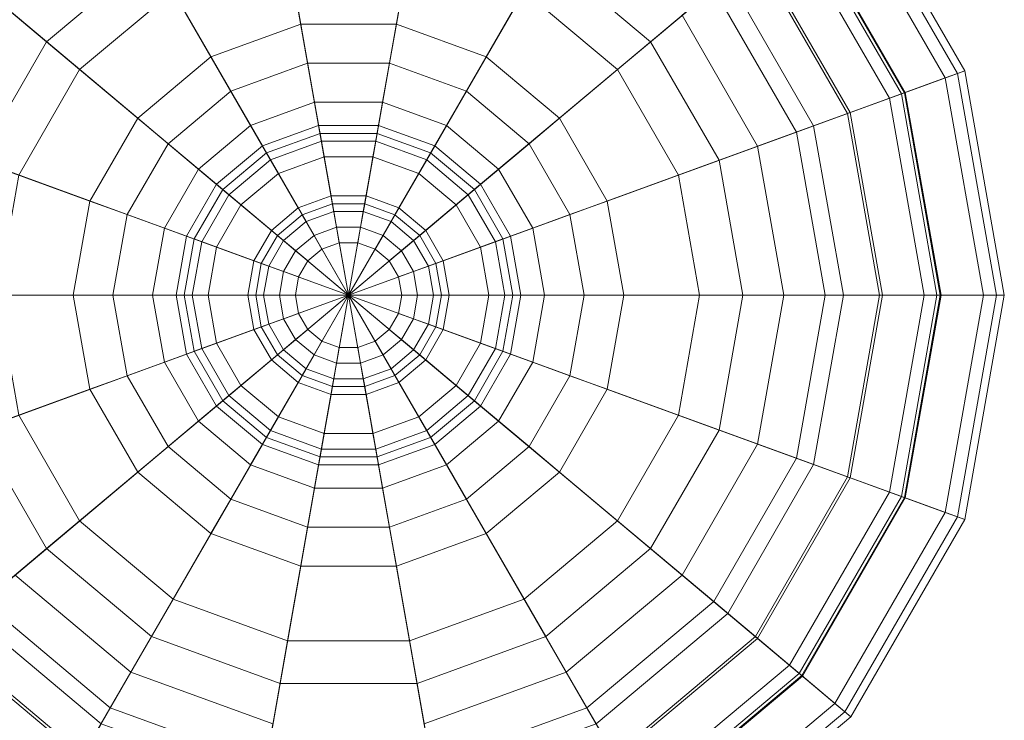
# Model space of a CAD drawing. Units: inches. Extents: x 375 to 1122, y 27 to 1069.
# Tile 22 of 155: x 718.584 to 720.617, y 272.362 to 273.809. Entities that reach past the tile are written whole.
import ezdxf

# ---------------------------------------------------------------- set-up
doc = ezdxf.new("R2010")
doc.units = ezdxf.units.IN
doc.layers.add('Furniture', color=30, linetype='Continuous', lineweight=18)

# ---------------------------------------------------------------- blocks, each defined once
blk = doc.blocks.new('A$C403C54AD')
for points in [[(1.826559, 0.891746, -0.031825), (1.826559, 0.857884, -0.028747), (1.826559, 0.857884, -0.028747), (1.814977, 0.889704, -0.031825)], [(1.826559, 0.88848, -0.028594), (1.826559, 0.891746, -0.031825), (1.814977, 0.889704, -0.031825), (1.816094, 0.886635, -0.028594)], [(1.826559, 0.88844, 0.131159), (1.826559, 0.891347, 0.117935), (1.815114, 0.889329, 0.117935), (1.816108, 0.886597, 0.131159)], [(1.826559, 0.891347, 0.117935), (1.826559, 0.890672, 0.089693), (1.815345, 0.888695, 0.089693), (1.815114, 0.889329, 0.117935)], [(1.83814, 0.889704, -0.031825), (1.826559, 0.857884, -0.028747), (1.826559, 0.857884, -0.028747), (1.826559, 0.891746, -0.031825)], [(1.837023, 0.886635, -0.028594), (1.83814, 0.889704, -0.031825), (1.826559, 0.891746, -0.031825), (1.826559, 0.88848, -0.028594)], [(1.83701, 0.886597, 0.131159), (1.838004, 0.889329, 0.117935), (1.826559, 0.891347, 0.117935), (1.826559, 0.88844, 0.131159)], [(1.838004, 0.889329, 0.117935), (1.837773, 0.888695, 0.089693), (1.826559, 0.890672, 0.089693), (1.826559, 0.891347, 0.117935)], [(1.826559, 0.890672, 0.089693), (1.826559, 0.885308, 0.071684), (1.817179, 0.883654, 0.071684), (1.815345, 0.888695, 0.089693)], [(1.837773, 0.888695, 0.089693), (1.835938, 0.883654, 0.071684), (1.826559, 0.885308, 0.071684), (1.826559, 0.890672, 0.089693)], [(1.816094, 0.886635, -0.028594), (1.814977, 0.889704, -0.031825), (1.804793, 0.883824, -0.031825), (1.806892, 0.881322, -0.028594)], [(1.814977, 0.889704, -0.031825), (1.826559, 0.857884, -0.028747), (1.826559, 0.857884, -0.028747), (1.804793, 0.883824, -0.031825)], [(1.816108, 0.886597, 0.131159), (1.815114, 0.889329, 0.117935), (1.805049, 0.883518, 0.117935), (1.806918, 0.881291, 0.131159)], [(1.815114, 0.889329, 0.117935), (1.815345, 0.888695, 0.089693), (1.805483, 0.883001, 0.089693), (1.805049, 0.883518, 0.117935)], [(1.848325, 0.883824, -0.031825), (1.826559, 0.857884, -0.028747), (1.826559, 0.857884, -0.028747), (1.83814, 0.889704, -0.031825)], [(1.8462, 0.881291, 0.131159), (1.848069, 0.883518, 0.117935), (1.838004, 0.889329, 0.117935), (1.83701, 0.886597, 0.131159)], [(1.846226, 0.881322, -0.028594), (1.848325, 0.883824, -0.031825), (1.83814, 0.889704, -0.031825), (1.837023, 0.886635, -0.028594)], [(1.848069, 0.883518, 0.117935), (1.847635, 0.883001, 0.089693), (1.837773, 0.888695, 0.089693), (1.838004, 0.889329, 0.117935)], [(1.815345, 0.888695, 0.089693), (1.817179, 0.883654, 0.071684), (1.808931, 0.878892, 0.071684), (1.805483, 0.883001, 0.089693)], [(1.826559, 0.872098, -0.02532), (1.826559, 0.88848, -0.028594), (1.816094, 0.886635, -0.028594), (1.821697, 0.871241, -0.02532)], [(1.826559, 0.883444, 0.140564), (1.826559, 0.88844, 0.131159), (1.816108, 0.886597, 0.131159), (1.817817, 0.881902, 0.140564)], [(1.826559, 0.888263, 0.117718), (1.826559, 0.885453, 0.130354), (1.81713, 0.88379, 0.130354), (1.816169, 0.886431, 0.117718)], [(1.826559, 0.887605, 0.090178), (1.826559, 0.888263, 0.117718), (1.816169, 0.886431, 0.117718), (1.816394, 0.885812, 0.090178)], [(1.83142, 0.871241, -0.02532), (1.837023, 0.886635, -0.028594), (1.826559, 0.88848, -0.028594), (1.826559, 0.872098, -0.02532)], [(1.835301, 0.881902, 0.140564), (1.83701, 0.886597, 0.131159), (1.826559, 0.88844, 0.131159), (1.826559, 0.883444, 0.140564)], [(1.836949, 0.886431, 0.117718), (1.835988, 0.88379, 0.130354), (1.826559, 0.885453, 0.130354), (1.826559, 0.888263, 0.117718)], [(1.836724, 0.885812, 0.090178), (1.836949, 0.886431, 0.117718), (1.826559, 0.888263, 0.117718), (1.826559, 0.887605, 0.090178)], [(1.847635, 0.883001, 0.089693), (1.844187, 0.878892, 0.071684), (1.835938, 0.883654, 0.071684), (1.837773, 0.888695, 0.089693)], [(1.826559, 0.882497, 0.073031), (1.826559, 0.887605, 0.090178), (1.816394, 0.885812, 0.090178), (1.818141, 0.881013, 0.073031)], [(1.834977, 0.881013, 0.073031), (1.836724, 0.885812, 0.090178), (1.826559, 0.887605, 0.090178), (1.826559, 0.882497, 0.073031)], [(1.821697, 0.871241, -0.02532), (1.816094, 0.886635, -0.028594), (1.806892, 0.881322, -0.028594), (1.817422, 0.868773, -0.02532)], [(1.817817, 0.881902, 0.140564), (1.816108, 0.886597, 0.131159), (1.806918, 0.881291, 0.131159), (1.81013, 0.877464, 0.140564)], [(1.816169, 0.886431, 0.117718), (1.81713, 0.88379, 0.130354), (1.808838, 0.879003, 0.130354), (1.807032, 0.881156, 0.117718)], [(1.816394, 0.885812, 0.090178), (1.816169, 0.886431, 0.117718), (1.807032, 0.881156, 0.117718), (1.807455, 0.880651, 0.090178)], [(1.835696, 0.868773, -0.02532), (1.846226, 0.881322, -0.028594), (1.837023, 0.886635, -0.028594), (1.83142, 0.871241, -0.02532)], [(1.842988, 0.877464, 0.140564), (1.8462, 0.881291, 0.131159), (1.83701, 0.886597, 0.131159), (1.835301, 0.881902, 0.140564)], [(1.846086, 0.881156, 0.117718), (1.84428, 0.879003, 0.130354), (1.835988, 0.88379, 0.130354), (1.836949, 0.886431, 0.117718)], [(1.845663, 0.880651, 0.090178), (1.846086, 0.881156, 0.117718), (1.836949, 0.886431, 0.117718), (1.836724, 0.885812, 0.090178)], [(1.818141, 0.881013, 0.073031), (1.816394, 0.885812, 0.090178), (1.807455, 0.880651, 0.090178), (1.810738, 0.876739, 0.073031)], [(1.84238, 0.876739, 0.073031), (1.845663, 0.880651, 0.090178), (1.836724, 0.885812, 0.090178), (1.834977, 0.881013, 0.073031)], [(1.826559, 0.885453, 0.130354), (1.826559, 0.880365, 0.140564), (1.81887, 0.879009, 0.140564), (1.81713, 0.88379, 0.130354)], [(1.826559, 0.885308, 0.071684), (1.826559, 0.878242, 0.061451), (1.819596, 0.877014, 0.061451), (1.817179, 0.883654, 0.071684)], [(1.835988, 0.88379, 0.130354), (1.834248, 0.879009, 0.140564), (1.826559, 0.880365, 0.140564), (1.826559, 0.885453, 0.130354)], [(1.835938, 0.883654, 0.071684), (1.833522, 0.877014, 0.061451), (1.826559, 0.878242, 0.061451), (1.826559, 0.885308, 0.071684)], [(1.804793, 0.883824, -0.031825), (1.826559, 0.857884, -0.028747), (1.826559, 0.857884, -0.028747), (1.797233, 0.874815, -0.031825)], [(1.81713, 0.88379, 0.130354), (1.81887, 0.879009, 0.140564), (1.812108, 0.875106, 0.140564), (1.808838, 0.879003, 0.130354)], [(1.855884, 0.874815, -0.031825), (1.826559, 0.857884, -0.028747), (1.826559, 0.857884, -0.028747), (1.848325, 0.883824, -0.031825)], [(1.84428, 0.879003, 0.130354), (1.84101, 0.875106, 0.140564), (1.834248, 0.879009, 0.140564), (1.835988, 0.88379, 0.130354)], [(1.853056, 0.873182, -0.028594), (1.855884, 0.874815, -0.031825), (1.848325, 0.883824, -0.031825), (1.846226, 0.881322, -0.028594)], [(1.817179, 0.883654, 0.071684), (1.819596, 0.877014, 0.061451), (1.813473, 0.873479, 0.061451), (1.808931, 0.878892, 0.071684)], [(1.826559, 0.880365, 0.140564), (1.826559, 0.883444, 0.140564), (1.817817, 0.881902, 0.140564), (1.81887, 0.879009, 0.140564)], [(1.834248, 0.879009, 0.140564), (1.835301, 0.881902, 0.140564), (1.826559, 0.883444, 0.140564), (1.826559, 0.880365, 0.140564)], [(1.844187, 0.878892, 0.071684), (1.839644, 0.873479, 0.061451), (1.833522, 0.877014, 0.061451), (1.835938, 0.883654, 0.071684)], [(1.853021, 0.873162, 0.131159), (1.855539, 0.874616, 0.117935), (1.848069, 0.883518, 0.117935), (1.8462, 0.881291, 0.131159)], [(1.855539, 0.874616, 0.117935), (1.854954, 0.874278, 0.089693), (1.847635, 0.883001, 0.089693), (1.848069, 0.883518, 0.117935)], [(1.854954, 0.874278, 0.089693), (1.850309, 0.871596, 0.071684), (1.844187, 0.878892, 0.071684), (1.847635, 0.883001, 0.089693)], [(1.826559, 0.876011, 0.063639), (1.826559, 0.882497, 0.073031), (1.818141, 0.881013, 0.073031), (1.820359, 0.874918, 0.063639)], [(1.832759, 0.874918, 0.063639), (1.834977, 0.881013, 0.073031), (1.826559, 0.882497, 0.073031), (1.826559, 0.876011, 0.063639)], [(1.81887, 0.879009, 0.140564), (1.817817, 0.881902, 0.140564), (1.81013, 0.877464, 0.140564), (1.812108, 0.875106, 0.140564)], [(1.84101, 0.875106, 0.140564), (1.842988, 0.877464, 0.140564), (1.835301, 0.881902, 0.140564), (1.834248, 0.879009, 0.140564)], [(1.817422, 0.868773, -0.02532), (1.806892, 0.881322, -0.028594), (1.800062, 0.873182, -0.028594), (1.814249, 0.864991, -0.02532)], [(1.838869, 0.864991, -0.02532), (1.853056, 0.873182, -0.028594), (1.846226, 0.881322, -0.028594), (1.835696, 0.868773, -0.02532)], [(1.848694, 0.870664, 0.140564), (1.853021, 0.873162, 0.131159), (1.8462, 0.881291, 0.131159), (1.842988, 0.877464, 0.140564)], [(1.852868, 0.873073, 0.117718), (1.850434, 0.871669, 0.130354), (1.84428, 0.879003, 0.130354), (1.846086, 0.881156, 0.117718)], [(1.852298, 0.872744, 0.090178), (1.852868, 0.873073, 0.117718), (1.846086, 0.881156, 0.117718), (1.845663, 0.880651, 0.090178)], [(1.820359, 0.874918, 0.063639), (1.818141, 0.881013, 0.073031), (1.810738, 0.876739, 0.073031), (1.814907, 0.87177, 0.063639)], [(1.838211, 0.87177, 0.063639), (1.84238, 0.876739, 0.073031), (1.834977, 0.881013, 0.073031), (1.832759, 0.874918, 0.063639)], [(1.847874, 0.87019, 0.073031), (1.852298, 0.872744, 0.090178), (1.845663, 0.880651, 0.090178), (1.84238, 0.876739, 0.073031)], [(1.808931, 0.878892, 0.071684), (1.813473, 0.873479, 0.061451), (1.808929, 0.868063, 0.061451), (1.802809, 0.871596, 0.071684)], [(1.850309, 0.871596, 0.071684), (1.844189, 0.868063, 0.061451), (1.839644, 0.873479, 0.061451), (1.844187, 0.878892, 0.071684)], [(1.850434, 0.871669, 0.130354), (1.846028, 0.869125, 0.140564), (1.84101, 0.875106, 0.140564), (1.84428, 0.879003, 0.130354)], [(1.826559, 0.878242, 0.061451), (1.826559, 0.868003, 0.054084), (1.823098, 0.867392, 0.054084), (1.819596, 0.877014, 0.061451)], [(1.833522, 0.877014, 0.061451), (1.83002, 0.867392, 0.054084), (1.826559, 0.868003, 0.054084), (1.826559, 0.878242, 0.061451)], [(1.846028, 0.869125, 0.140564), (1.848694, 0.870664, 0.140564), (1.842988, 0.877464, 0.140564), (1.84101, 0.875106, 0.140564)], [(1.814907, 0.87177, 0.063639), (1.810738, 0.876739, 0.073031), (1.805243, 0.87019, 0.073031), (1.81086, 0.866948, 0.063639)], [(1.819596, 0.877014, 0.061451), (1.823098, 0.867392, 0.054084), (1.820055, 0.865635, 0.054084), (1.813473, 0.873479, 0.061451)], [(1.839644, 0.873479, 0.061451), (1.833063, 0.865635, 0.054084), (1.83002, 0.867392, 0.054084), (1.833522, 0.877014, 0.061451)], [(1.842258, 0.866948, 0.063639), (1.847874, 0.87019, 0.073031), (1.84238, 0.876739, 0.073031), (1.838211, 0.87177, 0.063639)], [(1.826559, 0.866788, 0.057003), (1.826559, 0.876011, 0.063639), (1.820359, 0.874918, 0.063639), (1.823514, 0.866251, 0.057003)], [(1.829604, 0.866251, 0.057003), (1.832759, 0.874918, 0.063639), (1.826559, 0.876011, 0.063639), (1.826559, 0.866788, 0.057003)], [(1.797233, 0.874815, -0.031825), (1.826559, 0.857884, -0.028747), (1.826559, 0.857884, -0.028747), (1.793211, 0.863764, -0.031825)], [(1.823514, 0.866251, 0.057003), (1.820359, 0.874918, 0.063639), (1.814907, 0.87177, 0.063639), (1.820835, 0.864705, 0.057003)], [(1.859907, 0.863764, -0.031825), (1.826559, 0.857884, -0.028747), (1.826559, 0.857884, -0.028747), (1.855884, 0.874815, -0.031825)], [(1.832282, 0.864705, 0.057003), (1.838211, 0.87177, 0.063639), (1.832759, 0.874918, 0.063639), (1.829604, 0.866251, 0.057003)], [(1.814249, 0.864991, -0.02532), (1.800062, 0.873182, -0.028594), (1.796427, 0.863197, -0.028594), (1.812561, 0.860352, -0.02532)], [(1.813473, 0.873479, 0.061451), (1.820055, 0.865635, 0.054084), (1.817796, 0.862943, 0.054084), (1.808929, 0.868063, 0.061451)], [(1.844189, 0.868063, 0.061451), (1.835322, 0.862943, 0.054084), (1.833063, 0.865635, 0.054084), (1.839644, 0.873479, 0.061451)], [(1.840557, 0.860352, -0.02532), (1.85669, 0.863197, -0.028594), (1.853056, 0.873182, -0.028594), (1.838869, 0.864991, -0.02532)], [(1.850798, 0.862158, 0.073031), (1.855828, 0.863045, 0.090178), (1.852298, 0.872744, 0.090178), (1.847874, 0.87019, 0.073031)], [(1.826559, 0.87005, -0.022455), (1.826559, 0.872098, -0.02532), (1.821697, 0.871241, -0.02532), (1.822398, 0.869317, -0.022455)], [(1.83072, 0.869317, -0.022455), (1.83142, 0.871241, -0.02532), (1.826559, 0.872098, -0.02532), (1.826559, 0.87005, -0.022455)], [(1.820835, 0.864705, 0.057003), (1.814907, 0.87177, 0.063639), (1.81086, 0.866948, 0.063639), (1.818848, 0.862336, 0.057003)], [(1.83427, 0.862336, 0.057003), (1.842258, 0.866948, 0.063639), (1.838211, 0.87177, 0.063639), (1.832282, 0.864705, 0.057003)], [(1.853566, 0.862646, 0.071684), (1.846607, 0.861419, 0.061451), (1.844189, 0.868063, 0.061451), (1.850309, 0.871596, 0.071684)], [(1.853709, 0.862671, 0.130354), (1.848699, 0.861788, 0.140564), (1.846028, 0.869125, 0.140564), (1.850434, 0.871669, 0.130354)], [(1.822398, 0.869317, -0.022455), (1.821697, 0.871241, -0.02532), (1.817422, 0.868773, -0.02532), (1.818738, 0.867204, -0.022455)], [(1.834379, 0.867204, -0.022455), (1.835696, 0.868773, -0.02532), (1.83142, 0.871241, -0.02532), (1.83072, 0.869317, -0.022455)], [(1.848699, 0.861788, 0.140564), (1.85173, 0.862322, 0.140564), (1.848694, 0.870664, 0.140564), (1.846028, 0.869125, 0.140564)], [(1.826559, 0.865955, -0.020408), (1.826559, 0.87005, -0.022455), (1.822398, 0.869317, -0.022455), (1.823798, 0.865468, -0.020408)], [(1.829319, 0.865468, -0.020408), (1.83072, 0.869317, -0.022455), (1.826559, 0.87005, -0.022455), (1.826559, 0.865955, -0.020408)], [(1.844411, 0.861032, 0.063639), (1.850798, 0.862158, 0.073031), (1.847874, 0.87019, 0.073031), (1.842258, 0.866948, 0.063639)], [(1.823798, 0.865468, -0.020408), (1.822398, 0.869317, -0.022455), (1.818738, 0.867204, -0.022455), (1.821371, 0.864067, -0.020408)], [(1.831747, 0.864067, -0.020408), (1.834379, 0.867204, -0.022455), (1.83072, 0.869317, -0.022455), (1.829319, 0.865468, -0.020408)], [(1.818738, 0.867204, -0.022455), (1.817422, 0.868773, -0.02532), (1.814249, 0.864991, -0.02532), (1.816022, 0.863967, -0.022455)], [(1.837095, 0.863967, -0.022455), (1.838869, 0.864991, -0.02532), (1.835696, 0.868773, -0.02532), (1.834379, 0.867204, -0.022455)], [(1.808929, 0.868063, 0.061451), (1.817796, 0.862943, 0.054084), (1.816594, 0.859641, 0.054084), (1.806511, 0.861419, 0.061451)], [(1.826559, 0.868003, 0.054084), (1.826559, 0.863088, 0.053266), (1.824779, 0.862774, 0.053266), (1.823098, 0.867392, 0.054084)], [(1.83002, 0.867392, 0.054084), (1.828339, 0.862774, 0.053266), (1.826559, 0.863088, 0.053266), (1.826559, 0.868003, 0.054084)], [(1.846607, 0.861419, 0.061451), (1.836524, 0.859641, 0.054084), (1.835322, 0.862943, 0.054084), (1.844189, 0.868063, 0.061451)], [(1.818848, 0.862336, 0.057003), (1.81086, 0.866948, 0.063639), (1.808707, 0.861032, 0.063639), (1.81779, 0.85943, 0.057003)], [(1.821371, 0.864067, -0.020408), (1.818738, 0.867204, -0.022455), (1.816022, 0.863967, -0.022455), (1.819569, 0.861919, -0.020408)], [(1.823098, 0.867392, 0.054084), (1.824779, 0.862774, 0.053266), (1.823214, 0.861871, 0.053266), (1.820055, 0.865635, 0.054084)], [(1.833063, 0.865635, 0.054084), (1.829904, 0.861871, 0.053266), (1.828339, 0.862774, 0.053266), (1.83002, 0.867392, 0.054084)], [(1.833549, 0.861919, -0.020408), (1.837095, 0.863967, -0.022455), (1.834379, 0.867204, -0.022455), (1.831747, 0.864067, -0.020408)], [(1.835328, 0.85943, 0.057003), (1.844411, 0.861032, 0.063639), (1.842258, 0.866948, 0.063639), (1.83427, 0.862336, 0.057003)], [(1.826559, 0.857884, 0.055519), (1.826559, 0.866788, 0.057003), (1.823514, 0.866251, 0.057003), (1.826559, 0.857884, 0.055519)], [(1.826559, 0.857884, 0.055519), (1.829604, 0.866251, 0.057003), (1.826559, 0.866788, 0.057003), (1.826559, 0.857884, 0.055519)], [(1.826559, 0.857884, 0.055519), (1.823514, 0.866251, 0.057003), (1.820835, 0.864705, 0.057003), (1.826559, 0.857884, 0.055519)], [(1.826559, 0.866365, 0.0504), (1.826559, 0.862269, 0.048354), (1.825059, 0.862005, 0.048354), (1.823658, 0.865853, 0.0504)], [(1.826559, 0.865136, 0.052447), (1.826559, 0.866365, 0.0504), (1.823658, 0.865853, 0.0504), (1.824079, 0.864699, 0.052447)], [(1.826559, 0.862679, -0.015087), (1.826559, 0.865955, -0.020408), (1.823798, 0.865468, -0.020408), (1.824919, 0.862389, -0.015087)], [(1.829459, 0.865853, 0.0504), (1.828059, 0.862005, 0.048354), (1.826559, 0.862269, 0.048354), (1.826559, 0.866365, 0.0504)], [(1.829039, 0.864699, 0.052447), (1.829459, 0.865853, 0.0504), (1.826559, 0.866365, 0.0504), (1.826559, 0.865136, 0.052447)], [(1.826559, 0.857884, 0.055519), (1.832282, 0.864705, 0.057003), (1.829604, 0.866251, 0.057003), (1.826559, 0.857884, 0.055519)], [(1.828199, 0.862389, -0.015087), (1.829319, 0.865468, -0.020408), (1.826559, 0.865955, -0.020408), (1.826559, 0.862679, -0.015087)], [(1.820055, 0.865635, 0.054084), (1.823214, 0.861871, 0.053266), (1.822052, 0.860486, 0.053266), (1.817796, 0.862943, 0.054084)], [(1.823658, 0.865853, 0.0504), (1.825059, 0.862005, 0.048354), (1.82374, 0.861243, 0.048354), (1.821108, 0.86438, 0.0504)], [(1.824079, 0.864699, 0.052447), (1.823658, 0.865853, 0.0504), (1.821108, 0.86438, 0.0504), (1.821897, 0.863439, 0.052447)], [(1.824919, 0.862389, -0.015087), (1.823798, 0.865468, -0.020408), (1.821371, 0.864067, -0.020408), (1.823477, 0.861557, -0.015087)], [(1.83201, 0.86438, 0.0504), (1.829378, 0.861243, 0.048354), (1.828059, 0.862005, 0.048354), (1.829459, 0.865853, 0.0504)], [(1.829641, 0.861557, -0.015087), (1.831747, 0.864067, -0.020408), (1.829319, 0.865468, -0.020408), (1.828199, 0.862389, -0.015087)], [(1.83122, 0.863439, 0.052447), (1.83201, 0.86438, 0.0504), (1.829459, 0.865853, 0.0504), (1.829039, 0.864699, 0.052447)], [(1.835322, 0.862943, 0.054084), (1.831066, 0.860486, 0.053266), (1.829904, 0.861871, 0.053266), (1.833063, 0.865635, 0.054084)], [(1.816022, 0.863967, -0.022455), (1.814249, 0.864991, -0.02532), (1.812561, 0.860352, -0.02532), (1.814577, 0.859997, -0.022455)], [(1.826559, 0.863088, 0.053266), (1.826559, 0.865136, 0.052447), (1.824079, 0.864699, 0.052447), (1.824779, 0.862774, 0.053266)], [(1.828339, 0.862774, 0.053266), (1.829039, 0.864699, 0.052447), (1.826559, 0.865136, 0.052447), (1.826559, 0.863088, 0.053266)], [(1.838541, 0.859997, -0.022455), (1.840557, 0.860352, -0.02532), (1.838869, 0.864991, -0.02532), (1.837095, 0.863967, -0.022455)], [(1.826559, 0.857884, 0.055519), (1.820835, 0.864705, 0.057003), (1.818848, 0.862336, 0.057003), (1.826559, 0.857884, 0.055519)], [(1.821108, 0.86438, 0.0504), (1.82374, 0.861243, 0.048354), (1.822761, 0.860076, 0.048354), (1.819215, 0.862124, 0.0504)], [(1.821897, 0.863439, 0.052447), (1.821108, 0.86438, 0.0504), (1.819215, 0.862124, 0.0504), (1.820279, 0.86151, 0.052447)], [(1.824779, 0.862774, 0.053266), (1.824079, 0.864699, 0.052447), (1.821897, 0.863439, 0.052447), (1.823214, 0.861871, 0.053266)], [(1.826559, 0.857884, 0.055519), (1.83427, 0.862336, 0.057003), (1.832282, 0.864705, 0.057003), (1.826559, 0.857884, 0.055519)], [(1.829904, 0.861871, 0.053266), (1.83122, 0.863439, 0.052447), (1.829039, 0.864699, 0.052447), (1.828339, 0.862774, 0.053266)], [(1.833903, 0.862124, 0.0504), (1.830356, 0.860076, 0.048354), (1.829378, 0.861243, 0.048354), (1.83201, 0.86438, 0.0504)], [(1.832839, 0.86151, 0.052447), (1.833903, 0.862124, 0.0504), (1.83201, 0.86438, 0.0504), (1.83122, 0.863439, 0.052447)], [(1.819569, 0.861919, -0.020408), (1.816022, 0.863967, -0.022455), (1.814577, 0.859997, -0.022455), (1.818611, 0.859285, -0.020408)], [(1.823477, 0.861557, -0.015087), (1.821371, 0.864067, -0.020408), (1.819569, 0.861919, -0.020408), (1.822407, 0.860281, -0.015087)], [(1.830711, 0.860281, -0.015087), (1.833549, 0.861919, -0.020408), (1.831747, 0.864067, -0.020408), (1.829641, 0.861557, -0.015087)], [(1.834507, 0.859285, -0.020408), (1.838541, 0.859997, -0.022455), (1.837095, 0.863967, -0.022455), (1.833549, 0.861919, -0.020408)], [(1.793211, 0.863764, -0.031825), (1.826559, 0.857884, -0.028747), (1.826559, 0.857884, -0.028747), (1.793211, 0.852004, -0.031825)], [(1.823214, 0.861871, 0.053266), (1.821897, 0.863439, 0.052447), (1.820279, 0.86151, 0.052447), (1.822052, 0.860486, 0.053266)], [(1.859907, 0.852004, -0.031825), (1.826559, 0.857884, -0.028747), (1.826559, 0.857884, -0.028747), (1.859907, 0.863764, -0.031825)], [(1.831066, 0.860486, 0.053266), (1.832839, 0.86151, 0.052447), (1.83122, 0.863439, 0.052447), (1.829904, 0.861871, 0.053266)], [(1.812561, 0.860352, -0.02532), (1.796427, 0.863197, -0.028594), (1.796427, 0.852571, -0.028594), (1.812561, 0.855416, -0.02532)], [(1.817796, 0.862943, 0.054084), (1.822052, 0.860486, 0.053266), (1.821434, 0.858788, 0.053266), (1.816594, 0.859641, 0.054084)], [(1.836524, 0.859641, 0.054084), (1.831684, 0.858788, 0.053266), (1.831066, 0.860486, 0.053266), (1.835322, 0.862943, 0.054084)], [(1.840557, 0.855416, -0.02532), (1.85669, 0.852571, -0.028594), (1.85669, 0.863197, -0.028594), (1.840557, 0.860352, -0.02532)], [(1.826559, 0.857884, 0.055519), (1.818848, 0.862336, 0.057003), (1.81779, 0.85943, 0.057003), (1.826559, 0.857884, 0.055519)], [(1.825339, 0.861235, -0.006492), (1.824919, 0.862389, -0.015087), (1.823477, 0.861557, -0.015087), (1.824267, 0.860616, -0.006492)], [(1.826559, 0.86145, -0.006492), (1.826559, 0.862679, -0.015087), (1.824919, 0.862389, -0.015087), (1.825339, 0.861235, -0.006492)], [(1.827779, 0.861235, -0.006492), (1.828199, 0.862389, -0.015087), (1.826559, 0.862679, -0.015087), (1.826559, 0.86145, -0.006492)], [(1.826559, 0.857884, 0.055519), (1.835328, 0.85943, 0.057003), (1.83427, 0.862336, 0.057003), (1.826559, 0.857884, 0.055519)], [(1.828851, 0.860616, -0.006492), (1.829641, 0.861557, -0.015087), (1.828199, 0.862389, -0.015087), (1.827779, 0.861235, -0.006492)], [(1.853566, 0.853122, 0.071684), (1.846607, 0.854349, 0.061451), (1.846607, 0.861419, 0.061451), (1.853566, 0.862646, 0.071684)], [(1.820279, 0.86151, 0.052447), (1.819215, 0.862124, 0.0504), (1.818207, 0.859357, 0.0504), (1.819417, 0.859143, 0.052447)], [(1.819215, 0.862124, 0.0504), (1.822761, 0.860076, 0.048354), (1.82224, 0.858645, 0.048354), (1.818207, 0.859357, 0.0504)], [(1.822407, 0.860281, -0.015087), (1.819569, 0.861919, -0.020408), (1.818611, 0.859285, -0.020408), (1.821837, 0.858717, -0.015087)], [(1.825059, 0.862005, 0.048354), (1.825619, 0.860465, 0.041805), (1.824793, 0.859988, 0.041805), (1.82374, 0.861243, 0.048354)], [(1.826559, 0.862269, 0.048354), (1.826559, 0.860631, 0.041805), (1.825619, 0.860465, 0.041805), (1.825059, 0.862005, 0.048354)], [(1.828059, 0.862005, 0.048354), (1.827498, 0.860465, 0.041805), (1.826559, 0.860631, 0.041805), (1.826559, 0.862269, 0.048354)], [(1.829378, 0.861243, 0.048354), (1.828325, 0.859988, 0.041805), (1.827498, 0.860465, 0.041805), (1.828059, 0.862005, 0.048354)], [(1.834911, 0.859357, 0.0504), (1.830877, 0.858645, 0.048354), (1.830356, 0.860076, 0.048354), (1.833903, 0.862124, 0.0504)], [(1.831281, 0.858717, -0.015087), (1.834507, 0.859285, -0.020408), (1.833549, 0.861919, -0.020408), (1.830711, 0.860281, -0.015087)], [(1.833701, 0.859143, 0.052447), (1.834911, 0.859357, 0.0504), (1.833903, 0.862124, 0.0504), (1.832839, 0.86151, 0.052447)], [(1.844411, 0.854736, 0.063639), (1.850798, 0.85361, 0.073031), (1.850798, 0.862158, 0.073031), (1.844411, 0.861032, 0.063639)], [(1.806511, 0.861419, 0.061451), (1.816594, 0.859641, 0.054084), (1.816594, 0.856127, 0.054084), (1.806511, 0.854349, 0.061451)], [(1.822052, 0.860486, 0.053266), (1.820279, 0.86151, 0.052447), (1.819417, 0.859143, 0.052447), (1.821434, 0.858788, 0.053266)], [(1.824267, 0.860616, -0.006492), (1.823477, 0.861557, -0.015087), (1.822407, 0.860281, -0.015087), (1.823471, 0.859667, -0.006492)], [(1.826559, 0.860631, 0.041805), (1.826559, 0.86145, -0.006492), (1.825339, 0.861235, -0.006492), (1.825619, 0.860465, 0.041805)], [(1.827498, 0.860465, 0.041805), (1.827779, 0.861235, -0.006492), (1.826559, 0.86145, -0.006492), (1.826559, 0.860631, 0.041805)], [(1.829647, 0.859667, -0.006492), (1.830711, 0.860281, -0.015087), (1.829641, 0.861557, -0.015087), (1.828851, 0.860616, -0.006492)], [(1.831684, 0.858788, 0.053266), (1.833701, 0.859143, 0.052447), (1.832839, 0.86151, 0.052447), (1.831066, 0.860486, 0.053266)], [(1.846607, 0.854349, 0.061451), (1.836524, 0.856127, 0.054084), (1.836524, 0.859641, 0.054084), (1.846607, 0.861419, 0.061451)], [(1.81779, 0.85943, 0.057003), (1.808707, 0.861032, 0.063639), (1.808707, 0.854736, 0.063639), (1.81779, 0.856338, 0.057003)], [(1.82374, 0.861243, 0.048354), (1.824793, 0.859988, 0.041805), (1.82418, 0.859257, 0.041805), (1.822761, 0.860076, 0.048354)], [(1.825619, 0.860465, 0.041805), (1.825339, 0.861235, -0.006492), (1.824267, 0.860616, -0.006492), (1.824793, 0.859988, 0.041805)], [(1.828325, 0.859988, 0.041805), (1.828851, 0.860616, -0.006492), (1.827779, 0.861235, -0.006492), (1.827498, 0.860465, 0.041805)], [(1.830356, 0.860076, 0.048354), (1.828938, 0.859257, 0.041805), (1.828325, 0.859988, 0.041805), (1.829378, 0.861243, 0.048354)], [(1.835328, 0.856338, 0.057003), (1.844411, 0.854736, 0.063639), (1.844411, 0.861032, 0.063639), (1.835328, 0.85943, 0.057003)], [(1.814577, 0.859997, -0.022455), (1.812561, 0.860352, -0.02532), (1.812561, 0.855416, -0.02532), (1.814577, 0.855771, -0.022455)], [(1.824793, 0.859988, 0.041805), (1.824267, 0.860616, -0.006492), (1.823471, 0.859667, -0.006492), (1.82418, 0.859257, 0.041805)], [(1.828938, 0.859257, 0.041805), (1.829647, 0.859667, -0.006492), (1.828851, 0.860616, -0.006492), (1.828325, 0.859988, 0.041805)], [(1.838541, 0.855771, -0.022455), (1.840557, 0.855416, -0.02532), (1.840557, 0.860352, -0.02532), (1.838541, 0.859997, -0.022455)], [(1.818611, 0.859285, -0.020408), (1.814577, 0.859997, -0.022455), (1.814577, 0.855771, -0.022455), (1.818611, 0.856482, -0.020408)], [(1.823471, 0.859667, -0.006492), (1.822407, 0.860281, -0.015087), (1.821837, 0.858717, -0.015087), (1.823047, 0.858503, -0.006492)], [(1.822761, 0.860076, 0.048354), (1.82418, 0.859257, 0.041805), (1.823854, 0.858361, 0.041805), (1.82224, 0.858645, 0.048354)], [(1.830877, 0.858645, 0.048354), (1.829264, 0.858361, 0.041805), (1.828938, 0.859257, 0.041805), (1.830356, 0.860076, 0.048354)], [(1.830071, 0.858503, -0.006492), (1.831281, 0.858717, -0.015087), (1.830711, 0.860281, -0.015087), (1.829647, 0.859667, -0.006492)], [(1.834507, 0.856482, -0.020408), (1.838541, 0.855771, -0.022455), (1.838541, 0.859997, -0.022455), (1.834507, 0.859285, -0.020408)], [(1.816594, 0.859641, 0.054084), (1.821434, 0.858788, 0.053266), (1.821434, 0.85698, 0.053266), (1.816594, 0.856127, 0.054084)], [(1.826559, 0.857884, 0.055519), (1.81779, 0.85943, 0.057003), (1.81779, 0.856338, 0.057003), (1.826559, 0.857884, 0.055519)], [(1.819417, 0.859143, 0.052447), (1.818207, 0.859357, 0.0504), (1.818207, 0.856411, 0.0504), (1.819417, 0.856625, 0.052447)], [(1.818207, 0.859357, 0.0504), (1.82224, 0.858645, 0.048354), (1.82224, 0.857123, 0.048354), (1.818207, 0.856411, 0.0504)], [(1.821837, 0.858717, -0.015087), (1.818611, 0.859285, -0.020408), (1.818611, 0.856482, -0.020408), (1.821837, 0.857051, -0.015087)], [(1.82418, 0.859257, 0.041805), (1.823471, 0.859667, -0.006492), (1.823047, 0.858503, -0.006492), (1.823854, 0.858361, 0.041805)], [(1.826559, 0.857884, 0.055519), (1.835328, 0.856338, 0.057003), (1.835328, 0.85943, 0.057003), (1.826559, 0.857884, 0.055519)], [(1.829264, 0.858361, 0.041805), (1.830071, 0.858503, -0.006492), (1.829647, 0.859667, -0.006492), (1.828938, 0.859257, 0.041805)], [(1.834911, 0.856411, 0.0504), (1.830877, 0.857123, 0.048354), (1.830877, 0.858645, 0.048354), (1.834911, 0.859357, 0.0504)], [(1.831281, 0.857051, -0.015087), (1.834507, 0.856482, -0.020408), (1.834507, 0.859285, -0.020408), (1.831281, 0.858717, -0.015087)], [(1.836524, 0.856127, 0.054084), (1.831684, 0.85698, 0.053266), (1.831684, 0.858788, 0.053266), (1.836524, 0.859641, 0.054084)], [(1.833701, 0.856625, 0.052447), (1.834911, 0.856411, 0.0504), (1.834911, 0.859357, 0.0504), (1.833701, 0.859143, 0.052447)], [(1.821434, 0.858788, 0.053266), (1.819417, 0.859143, 0.052447), (1.819417, 0.856625, 0.052447), (1.821434, 0.85698, 0.053266)], [(1.831684, 0.85698, 0.053266), (1.833701, 0.856625, 0.052447), (1.833701, 0.859143, 0.052447), (1.831684, 0.858788, 0.053266)], [(1.823047, 0.858503, -0.006492), (1.821837, 0.858717, -0.015087), (1.821837, 0.857051, -0.015087), (1.823047, 0.857265, -0.006492)], [(1.82224, 0.858645, 0.048354), (1.823854, 0.858361, 0.041805), (1.823854, 0.857407, 0.041805), (1.82224, 0.857123, 0.048354)], [(1.823854, 0.858361, 0.041805), (1.823047, 0.858503, -0.006492), (1.823047, 0.857265, -0.006492), (1.823854, 0.857407, 0.041805)], [(1.830877, 0.857123, 0.048354), (1.829264, 0.857407, 0.041805), (1.829264, 0.858361, 0.041805), (1.830877, 0.858645, 0.048354)], [(1.829264, 0.857407, 0.041805), (1.830071, 0.857265, -0.006492), (1.830071, 0.858503, -0.006492), (1.829264, 0.858361, 0.041805)], [(1.830071, 0.857265, -0.006492), (1.831281, 0.857051, -0.015087), (1.831281, 0.858717, -0.015087), (1.830071, 0.858503, -0.006492)], [(1.793211, 0.852004, -0.031825), (1.826559, 0.857884, -0.028747), (1.826559, 0.857884, -0.028747), (1.797233, 0.840953, -0.031825)], [(1.797233, 0.840953, -0.031825), (1.826559, 0.857884, -0.028747), (1.826559, 0.857884, -0.028747), (1.804793, 0.831944, -0.031825)], [(1.804793, 0.831944, -0.031825), (1.826559, 0.857884, -0.028747), (1.826559, 0.857884, -0.028747), (1.814977, 0.826064, -0.031825)], [(1.814977, 0.826064, -0.031825), (1.826559, 0.857884, -0.028747), (1.826559, 0.857884, -0.028747), (1.826559, 0.824022, -0.031825)], [(1.826559, 0.857884, 0.055519), (1.81779, 0.856338, 0.057003), (1.818848, 0.853432, 0.057003), (1.826559, 0.857884, 0.055519)], [(1.826559, 0.857884, 0.055519), (1.818848, 0.853432, 0.057003), (1.820835, 0.851063, 0.057003), (1.826559, 0.857884, 0.055519)], [(1.826559, 0.857884, 0.055519), (1.820835, 0.851063, 0.057003), (1.823514, 0.849517, 0.057003), (1.826559, 0.857884, 0.055519)], [(1.826559, 0.857884, 0.055519), (1.823514, 0.849517, 0.057003), (1.826559, 0.84898, 0.057003), (1.826559, 0.857884, 0.055519)], [(1.826559, 0.857884, 0.055519), (1.83427, 0.853432, 0.057003), (1.835328, 0.856338, 0.057003), (1.826559, 0.857884, 0.055519)], [(1.826559, 0.857884, 0.055519), (1.832282, 0.851063, 0.057003), (1.83427, 0.853432, 0.057003), (1.826559, 0.857884, 0.055519)], [(1.826559, 0.857884, 0.055519), (1.829604, 0.849517, 0.057003), (1.832282, 0.851063, 0.057003), (1.826559, 0.857884, 0.055519)], [(1.826559, 0.857884, 0.055519), (1.826559, 0.84898, 0.057003), (1.829604, 0.849517, 0.057003), (1.826559, 0.857884, 0.055519)], [(1.855884, 0.840953, -0.031825), (1.826559, 0.857884, -0.028747), (1.826559, 0.857884, -0.028747), (1.859907, 0.852004, -0.031825)], [(1.848325, 0.831944, -0.031825), (1.826559, 0.857884, -0.028747), (1.826559, 0.857884, -0.028747), (1.855884, 0.840953, -0.031825)], [(1.83814, 0.826064, -0.031825), (1.826559, 0.857884, -0.028747), (1.826559, 0.857884, -0.028747), (1.848325, 0.831944, -0.031825)], [(1.826559, 0.824022, -0.031825), (1.826559, 0.857884, -0.028747), (1.826559, 0.857884, -0.028747), (1.83814, 0.826064, -0.031825)], [(1.823047, 0.857265, -0.006492), (1.821837, 0.857051, -0.015087), (1.822407, 0.855487, -0.015087), (1.823471, 0.856101, -0.006492)], [(1.82224, 0.857123, 0.048354), (1.823854, 0.857407, 0.041805), (1.82418, 0.856511, 0.041805), (1.822761, 0.855691, 0.048354)], [(1.823854, 0.857407, 0.041805), (1.823047, 0.857265, -0.006492), (1.823471, 0.856101, -0.006492), (1.82418, 0.856511, 0.041805)], [(1.830356, 0.855691, 0.048354), (1.828938, 0.856511, 0.041805), (1.829264, 0.857407, 0.041805), (1.830877, 0.857123, 0.048354)], [(1.828938, 0.856511, 0.041805), (1.829647, 0.856101, -0.006492), (1.830071, 0.857265, -0.006492), (1.829264, 0.857407, 0.041805)], [(1.829647, 0.856101, -0.006492), (1.830711, 0.855487, -0.015087), (1.831281, 0.857051, -0.015087), (1.830071, 0.857265, -0.006492)], [(1.816594, 0.856127, 0.054084), (1.821434, 0.85698, 0.053266), (1.822052, 0.855282, 0.053266), (1.817796, 0.852825, 0.054084)], [(1.818207, 0.856411, 0.0504), (1.82224, 0.857123, 0.048354), (1.822761, 0.855691, 0.048354), (1.819215, 0.853644, 0.0504)], [(1.821837, 0.857051, -0.015087), (1.818611, 0.856482, -0.020408), (1.819569, 0.853848, -0.020408), (1.822407, 0.855487, -0.015087)], [(1.821434, 0.85698, 0.053266), (1.819417, 0.856625, 0.052447), (1.820279, 0.854258, 0.052447), (1.822052, 0.855282, 0.053266)], [(1.833903, 0.853644, 0.0504), (1.830356, 0.855691, 0.048354), (1.830877, 0.857123, 0.048354), (1.834911, 0.856411, 0.0504)], [(1.830711, 0.855487, -0.015087), (1.833549, 0.853848, -0.020408), (1.834507, 0.856482, -0.020408), (1.831281, 0.857051, -0.015087)], [(1.831066, 0.855282, 0.053266), (1.832839, 0.854258, 0.052447), (1.833701, 0.856625, 0.052447), (1.831684, 0.85698, 0.053266)], [(1.835322, 0.852825, 0.054084), (1.831066, 0.855282, 0.053266), (1.831684, 0.85698, 0.053266), (1.836524, 0.856127, 0.054084)], [(1.81779, 0.856338, 0.057003), (1.808707, 0.854736, 0.063639), (1.81086, 0.84882, 0.063639), (1.818848, 0.853432, 0.057003)], [(1.818611, 0.856482, -0.020408), (1.814577, 0.855771, -0.022455), (1.816022, 0.851801, -0.022455), (1.819569, 0.853848, -0.020408)], [(1.819417, 0.856625, 0.052447), (1.818207, 0.856411, 0.0504), (1.819215, 0.853644, 0.0504), (1.820279, 0.854258, 0.052447)], [(1.822761, 0.855691, 0.048354), (1.82418, 0.856511, 0.041805), (1.824793, 0.85578, 0.041805), (1.82374, 0.854525, 0.048354)], [(1.82418, 0.856511, 0.041805), (1.823471, 0.856101, -0.006492), (1.824267, 0.855152, -0.006492), (1.824793, 0.85578, 0.041805)], [(1.829378, 0.854525, 0.048354), (1.828325, 0.85578, 0.041805), (1.828938, 0.856511, 0.041805), (1.830356, 0.855691, 0.048354)], [(1.828325, 0.85578, 0.041805), (1.828851, 0.855152, -0.006492), (1.829647, 0.856101, -0.006492), (1.828938, 0.856511, 0.041805)], [(1.832839, 0.854258, 0.052447), (1.833903, 0.853644, 0.0504), (1.834911, 0.856411, 0.0504), (1.833701, 0.856625, 0.052447)], [(1.833549, 0.853848, -0.020408), (1.837095, 0.851801, -0.022455), (1.838541, 0.855771, -0.022455), (1.834507, 0.856482, -0.020408)], [(1.83427, 0.853432, 0.057003), (1.842258, 0.84882, 0.063639), (1.844411, 0.854736, 0.063639), (1.835328, 0.856338, 0.057003)], [(1.806511, 0.854349, 0.061451), (1.816594, 0.856127, 0.054084), (1.817796, 0.852825, 0.054084), (1.808929, 0.847705, 0.061451)], [(1.814577, 0.855771, -0.022455), (1.812561, 0.855416, -0.02532), (1.814249, 0.850777, -0.02532), (1.816022, 0.851801, -0.022455)], [(1.823471, 0.856101, -0.006492), (1.822407, 0.855487, -0.015087), (1.823477, 0.854211, -0.015087), (1.824267, 0.855152, -0.006492)], [(1.82374, 0.854525, 0.048354), (1.824793, 0.85578, 0.041805), (1.825619, 0.855303, 0.041805), (1.825059, 0.853763, 0.048354)], [(1.824793, 0.85578, 0.041805), (1.824267, 0.855152, -0.006492), (1.825339, 0.854533, -0.006492), (1.825619, 0.855303, 0.041805)], [(1.828059, 0.853763, 0.048354), (1.827498, 0.855303, 0.041805), (1.828325, 0.85578, 0.041805), (1.829378, 0.854525, 0.048354)], [(1.827498, 0.855303, 0.041805), (1.827779, 0.854533, -0.006492), (1.828851, 0.855152, -0.006492), (1.828325, 0.85578, 0.041805)], [(1.828851, 0.855152, -0.006492), (1.829641, 0.854211, -0.015087), (1.830711, 0.855487, -0.015087), (1.829647, 0.856101, -0.006492)], [(1.844189, 0.847705, 0.061451), (1.835322, 0.852825, 0.054084), (1.836524, 0.856127, 0.054084), (1.846607, 0.854349, 0.061451)], [(1.837095, 0.851801, -0.022455), (1.838869, 0.850777, -0.02532), (1.840557, 0.855416, -0.02532), (1.838541, 0.855771, -0.022455)], [(1.812561, 0.855416, -0.02532), (1.796427, 0.852571, -0.028594), (1.800062, 0.842586, -0.028594), (1.814249, 0.850777, -0.02532)], [(1.817796, 0.852825, 0.054084), (1.822052, 0.855282, 0.053266), (1.823214, 0.853897, 0.053266), (1.820055, 0.850133, 0.054084)], [(1.819215, 0.853644, 0.0504), (1.822761, 0.855691, 0.048354), (1.82374, 0.854525, 0.048354), (1.821108, 0.851387, 0.0504)], [(1.822407, 0.855487, -0.015087), (1.819569, 0.853848, -0.020408), (1.821371, 0.851701, -0.020408), (1.823477, 0.854211, -0.015087)], [(1.822052, 0.855282, 0.053266), (1.820279, 0.854258, 0.052447), (1.821897, 0.852329, 0.052447), (1.823214, 0.853897, 0.053266)], [(1.825059, 0.853763, 0.048354), (1.825619, 0.855303, 0.041805), (1.826559, 0.855137, 0.041805), (1.826559, 0.853499, 0.048354)], [(1.825619, 0.855303, 0.041805), (1.825339, 0.854533, -0.006492), (1.826559, 0.854318, -0.006492), (1.826559, 0.855137, 0.041805)], [(1.826559, 0.853499, 0.048354), (1.826559, 0.855137, 0.041805), (1.827498, 0.855303, 0.041805), (1.828059, 0.853763, 0.048354)], [(1.826559, 0.855137, 0.041805), (1.826559, 0.854318, -0.006492), (1.827779, 0.854533, -0.006492), (1.827498, 0.855303, 0.041805)], [(1.83201, 0.851387, 0.0504), (1.829378, 0.854525, 0.048354), (1.830356, 0.855691, 0.048354), (1.833903, 0.853644, 0.0504)], [(1.829641, 0.854211, -0.015087), (1.831747, 0.851701, -0.020408), (1.833549, 0.853848, -0.020408), (1.830711, 0.855487, -0.015087)], [(1.829904, 0.853897, 0.053266), (1.83122, 0.852329, 0.052447), (1.832839, 0.854258, 0.052447), (1.831066, 0.855282, 0.053266)], [(1.833063, 0.850133, 0.054084), (1.829904, 0.853897, 0.053266), (1.831066, 0.855282, 0.053266), (1.835322, 0.852825, 0.054084)], [(1.838869, 0.850777, -0.02532), (1.853056, 0.842586, -0.028594), (1.85669, 0.852571, -0.028594), (1.840557, 0.855416, -0.02532)], [(1.824267, 0.855152, -0.006492), (1.823477, 0.854211, -0.015087), (1.824919, 0.853379, -0.015087), (1.825339, 0.854533, -0.006492)], [(1.827779, 0.854533, -0.006492), (1.828199, 0.853379, -0.015087), (1.829641, 0.854211, -0.015087), (1.828851, 0.855152, -0.006492)], [(1.842258, 0.84882, 0.063639), (1.847874, 0.845577, 0.073031), (1.850798, 0.85361, 0.073031), (1.844411, 0.854736, 0.063639)], [(1.820279, 0.854258, 0.052447), (1.819215, 0.853644, 0.0504), (1.821108, 0.851387, 0.0504), (1.821897, 0.852329, 0.052447)], [(1.821108, 0.851387, 0.0504), (1.82374, 0.854525, 0.048354), (1.825059, 0.853763, 0.048354), (1.823658, 0.849915, 0.0504)], [(1.823477, 0.854211, -0.015087), (1.821371, 0.851701, -0.020408), (1.823798, 0.8503, -0.020408), (1.824919, 0.853379, -0.015087)], [(1.825339, 0.854533, -0.006492), (1.824919, 0.853379, -0.015087), (1.826559, 0.853089, -0.015087), (1.826559, 0.854318, -0.006492)], [(1.826559, 0.854318, -0.006492), (1.826559, 0.853089, -0.015087), (1.828199, 0.853379, -0.015087), (1.827779, 0.854533, -0.006492)], [(1.829459, 0.849915, 0.0504), (1.828059, 0.853763, 0.048354), (1.829378, 0.854525, 0.048354), (1.83201, 0.851387, 0.0504)], [(1.828199, 0.853379, -0.015087), (1.829319, 0.8503, -0.020408), (1.831747, 0.851701, -0.020408), (1.829641, 0.854211, -0.015087)], [(1.83122, 0.852329, 0.052447), (1.83201, 0.851387, 0.0504), (1.833903, 0.853644, 0.0504), (1.832839, 0.854258, 0.052447)], [(1.850309, 0.844172, 0.071684), (1.844189, 0.847705, 0.061451), (1.846607, 0.854349, 0.061451), (1.853566, 0.853122, 0.071684)], [(1.819569, 0.853848, -0.020408), (1.816022, 0.851801, -0.022455), (1.818738, 0.848564, -0.022455), (1.821371, 0.851701, -0.020408)], [(1.820055, 0.850133, 0.054084), (1.823214, 0.853897, 0.053266), (1.824779, 0.852994, 0.053266), (1.823098, 0.848375, 0.054084)], [(1.823214, 0.853897, 0.053266), (1.821897, 0.852329, 0.052447), (1.824079, 0.851069, 0.052447), (1.824779, 0.852994, 0.053266)], [(1.823658, 0.849915, 0.0504), (1.825059, 0.853763, 0.048354), (1.826559, 0.853499, 0.048354), (1.826559, 0.849403, 0.0504)], [(1.826559, 0.849403, 0.0504), (1.826559, 0.853499, 0.048354), (1.828059, 0.853763, 0.048354), (1.829459, 0.849915, 0.0504)], [(1.828339, 0.852994, 0.053266), (1.829039, 0.851069, 0.052447), (1.83122, 0.852329, 0.052447), (1.829904, 0.853897, 0.053266)], [(1.83002, 0.848375, 0.054084), (1.828339, 0.852994, 0.053266), (1.829904, 0.853897, 0.053266), (1.833063, 0.850133, 0.054084)], [(1.831747, 0.851701, -0.020408), (1.834379, 0.848564, -0.022455), (1.837095, 0.851801, -0.022455), (1.833549, 0.853848, -0.020408)], [(1.846028, 0.846643, 0.140564), (1.848694, 0.845104, 0.140564), (1.85173, 0.853446, 0.140564), (1.848699, 0.85398, 0.140564)], [(1.850434, 0.844099, 0.130354), (1.846028, 0.846643, 0.140564), (1.848699, 0.85398, 0.140564), (1.853709, 0.853097, 0.130354)], [(1.818848, 0.853432, 0.057003), (1.81086, 0.84882, 0.063639), (1.814907, 0.843998, 0.063639), (1.820835, 0.851063, 0.057003)], [(1.824919, 0.853379, -0.015087), (1.823798, 0.8503, -0.020408), (1.826559, 0.849813, -0.020408), (1.826559, 0.853089, -0.015087)], [(1.826559, 0.853089, -0.015087), (1.826559, 0.849813, -0.020408), (1.829319, 0.8503, -0.020408), (1.828199, 0.853379, -0.015087)], [(1.832282, 0.851063, 0.057003), (1.838211, 0.843998, 0.063639), (1.842258, 0.84882, 0.063639), (1.83427, 0.853432, 0.057003)], [(1.847874, 0.845577, 0.073031), (1.852298, 0.843024, 0.090178), (1.855828, 0.852723, 0.090178), (1.850798, 0.85361, 0.073031)], [(1.808929, 0.847705, 0.061451), (1.817796, 0.852825, 0.054084), (1.820055, 0.850133, 0.054084), (1.813473, 0.842289, 0.061451)], [(1.823098, 0.848375, 0.054084), (1.824779, 0.852994, 0.053266), (1.826559, 0.85268, 0.053266), (1.826559, 0.847765, 0.054084)], [(1.824779, 0.852994, 0.053266), (1.824079, 0.851069, 0.052447), (1.826559, 0.850632, 0.052447), (1.826559, 0.85268, 0.053266)], [(1.826559, 0.85268, 0.053266), (1.826559, 0.850632, 0.052447), (1.829039, 0.851069, 0.052447), (1.828339, 0.852994, 0.053266)], [(1.826559, 0.847765, 0.054084), (1.826559, 0.85268, 0.053266), (1.828339, 0.852994, 0.053266), (1.83002, 0.848375, 0.054084)], [(1.839644, 0.842289, 0.061451), (1.833063, 0.850133, 0.054084), (1.835322, 0.852825, 0.054084), (1.844189, 0.847705, 0.061451)], [(1.821897, 0.852329, 0.052447), (1.821108, 0.851387, 0.0504), (1.823658, 0.849915, 0.0504), (1.824079, 0.851069, 0.052447)], [(1.829039, 0.851069, 0.052447), (1.829459, 0.849915, 0.0504), (1.83201, 0.851387, 0.0504), (1.83122, 0.852329, 0.052447)], [(1.816022, 0.851801, -0.022455), (1.814249, 0.850777, -0.02532), (1.817422, 0.846995, -0.02532), (1.818738, 0.848564, -0.022455)], [(1.821371, 0.851701, -0.020408), (1.818738, 0.848564, -0.022455), (1.822398, 0.846451, -0.022455), (1.823798, 0.8503, -0.020408)], [(1.829319, 0.8503, -0.020408), (1.83072, 0.846451, -0.022455), (1.834379, 0.848564, -0.022455), (1.831747, 0.851701, -0.020408)], [(1.834379, 0.848564, -0.022455), (1.835696, 0.846995, -0.02532), (1.838869, 0.850777, -0.02532), (1.837095, 0.851801, -0.022455)], [(1.814249, 0.850777, -0.02532), (1.800062, 0.842586, -0.028594), (1.806892, 0.834446, -0.028594), (1.817422, 0.846995, -0.02532)], [(1.820835, 0.851063, 0.057003), (1.814907, 0.843998, 0.063639), (1.820359, 0.84085, 0.063639), (1.823514, 0.849517, 0.057003)], [(1.824079, 0.851069, 0.052447), (1.823658, 0.849915, 0.0504), (1.826559, 0.849403, 0.0504), (1.826559, 0.850632, 0.052447)], [(1.826559, 0.850632, 0.052447), (1.826559, 0.849403, 0.0504), (1.829459, 0.849915, 0.0504), (1.829039, 0.851069, 0.052447)], [(1.829604, 0.849517, 0.057003), (1.832759, 0.84085, 0.063639), (1.838211, 0.843998, 0.063639), (1.832282, 0.851063, 0.057003)], [(1.835696, 0.846995, -0.02532), (1.846226, 0.834446, -0.028594), (1.853056, 0.842586, -0.028594), (1.838869, 0.850777, -0.02532)], [(1.813473, 0.842289, 0.061451), (1.820055, 0.850133, 0.054084), (1.823098, 0.848375, 0.054084), (1.819596, 0.838754, 0.061451)], [(1.823798, 0.8503, -0.020408), (1.822398, 0.846451, -0.022455), (1.826559, 0.845717, -0.022455), (1.826559, 0.849813, -0.020408)], [(1.826559, 0.849813, -0.020408), (1.826559, 0.845717, -0.022455), (1.83072, 0.846451, -0.022455), (1.829319, 0.8503, -0.020408)], [(1.833522, 0.838754, 0.061451), (1.83002, 0.848375, 0.054084), (1.833063, 0.850133, 0.054084), (1.839644, 0.842289, 0.061451)], [(1.823514, 0.849517, 0.057003), (1.820359, 0.84085, 0.063639), (1.826559, 0.839757, 0.063639), (1.826559, 0.84898, 0.057003)], [(1.826559, 0.84898, 0.057003), (1.826559, 0.839757, 0.063639), (1.832759, 0.84085, 0.063639), (1.829604, 0.849517, 0.057003)], [(1.81086, 0.84882, 0.063639), (1.805243, 0.845577, 0.073031), (1.810738, 0.839029, 0.073031), (1.814907, 0.843998, 0.063639)], [(1.838211, 0.843998, 0.063639), (1.84238, 0.839029, 0.073031), (1.847874, 0.845577, 0.073031), (1.842258, 0.84882, 0.063639)], [(1.818738, 0.848564, -0.022455), (1.817422, 0.846995, -0.02532), (1.821697, 0.844527, -0.02532), (1.822398, 0.846451, -0.022455)], [(1.819596, 0.838754, 0.061451), (1.823098, 0.848375, 0.054084), (1.826559, 0.847765, 0.054084), (1.826559, 0.837526, 0.061451)], [(1.826559, 0.837526, 0.061451), (1.826559, 0.847765, 0.054084), (1.83002, 0.848375, 0.054084), (1.833522, 0.838754, 0.061451)], [(1.83072, 0.846451, -0.022455), (1.83142, 0.844527, -0.02532), (1.835696, 0.846995, -0.02532), (1.834379, 0.848564, -0.022455)], [(1.802809, 0.844172, 0.071684), (1.808929, 0.847705, 0.061451), (1.813473, 0.842289, 0.061451), (1.808931, 0.836876, 0.071684)], [(1.844187, 0.836876, 0.071684), (1.839644, 0.842289, 0.061451), (1.844189, 0.847705, 0.061451), (1.850309, 0.844172, 0.071684)], [(1.817422, 0.846995, -0.02532), (1.806892, 0.834446, -0.028594), (1.816094, 0.829133, -0.028594), (1.821697, 0.844527, -0.02532)], [(1.83142, 0.844527, -0.02532), (1.837023, 0.829133, -0.028594), (1.846226, 0.834446, -0.028594), (1.835696, 0.846995, -0.02532)], [(1.84101, 0.840662, 0.140564), (1.842988, 0.838304, 0.140564), (1.848694, 0.845104, 0.140564), (1.846028, 0.846643, 0.140564)], [(1.84428, 0.836765, 0.130354), (1.84101, 0.840662, 0.140564), (1.846028, 0.846643, 0.140564), (1.850434, 0.844099, 0.130354)], [(1.822398, 0.846451, -0.022455), (1.821697, 0.844527, -0.02532), (1.826559, 0.84367, -0.02532), (1.826559, 0.845717, -0.022455)], [(1.826559, 0.845717, -0.022455), (1.826559, 0.84367, -0.02532), (1.83142, 0.844527, -0.02532), (1.83072, 0.846451, -0.022455)], [(1.84238, 0.839029, 0.073031), (1.845663, 0.835117, 0.090178), (1.852298, 0.843024, 0.090178), (1.847874, 0.845577, 0.073031)], [(1.842988, 0.838304, 0.140564), (1.8462, 0.834477, 0.131159), (1.853021, 0.842606, 0.131159), (1.848694, 0.845104, 0.140564)], [(1.821697, 0.844527, -0.02532), (1.816094, 0.829133, -0.028594), (1.826559, 0.827288, -0.028594), (1.826559, 0.84367, -0.02532)], [(1.826559, 0.84367, -0.02532), (1.826559, 0.827288, -0.028594), (1.837023, 0.829133, -0.028594), (1.83142, 0.844527, -0.02532)], [(1.847635, 0.832767, 0.089693), (1.844187, 0.836876, 0.071684), (1.850309, 0.844172, 0.071684), (1.854954, 0.84149, 0.089693)], [(1.846086, 0.834612, 0.117718), (1.84428, 0.836765, 0.130354), (1.850434, 0.844099, 0.130354), (1.852868, 0.842695, 0.117718)], [(1.814907, 0.843998, 0.063639), (1.810738, 0.839029, 0.073031), (1.818141, 0.834755, 0.073031), (1.820359, 0.84085, 0.063639)], [(1.832759, 0.84085, 0.063639), (1.834977, 0.834755, 0.073031), (1.84238, 0.839029, 0.073031), (1.838211, 0.843998, 0.063639)], [(1.845663, 0.835117, 0.090178), (1.846086, 0.834612, 0.117718), (1.852868, 0.842695, 0.117718), (1.852298, 0.843024, 0.090178)], [(1.8462, 0.834477, 0.131159), (1.848069, 0.83225, 0.117935), (1.855539, 0.841152, 0.117935), (1.853021, 0.842606, 0.131159)], [(1.846226, 0.834446, -0.028594), (1.848325, 0.831944, -0.031825), (1.855884, 0.840953, -0.031825), (1.853056, 0.842586, -0.028594)], [(1.808931, 0.836876, 0.071684), (1.813473, 0.842289, 0.061451), (1.819596, 0.838754, 0.061451), (1.817179, 0.832114, 0.071684)], [(1.835938, 0.832114, 0.071684), (1.833522, 0.838754, 0.061451), (1.839644, 0.842289, 0.061451), (1.844187, 0.836876, 0.071684)], [(1.848069, 0.83225, 0.117935), (1.847635, 0.832767, 0.089693), (1.854954, 0.84149, 0.089693), (1.855539, 0.841152, 0.117935)]]:
    blk.add_3dface(points)

msp = doc.modelspace()

# ---------------------------------------------------------------- block references
at = {"layer": 'Furniture', "xscale": 39.9918517141215, "yscale": 39.9918517141215, "zscale": 39.9918517141215, "rotation": 270}
msp.add_blockref('A$C403C54AD', (684.9549, 346.2875, 0.024), dxfattribs=at)

doc.saveas('drawing.dxf')
